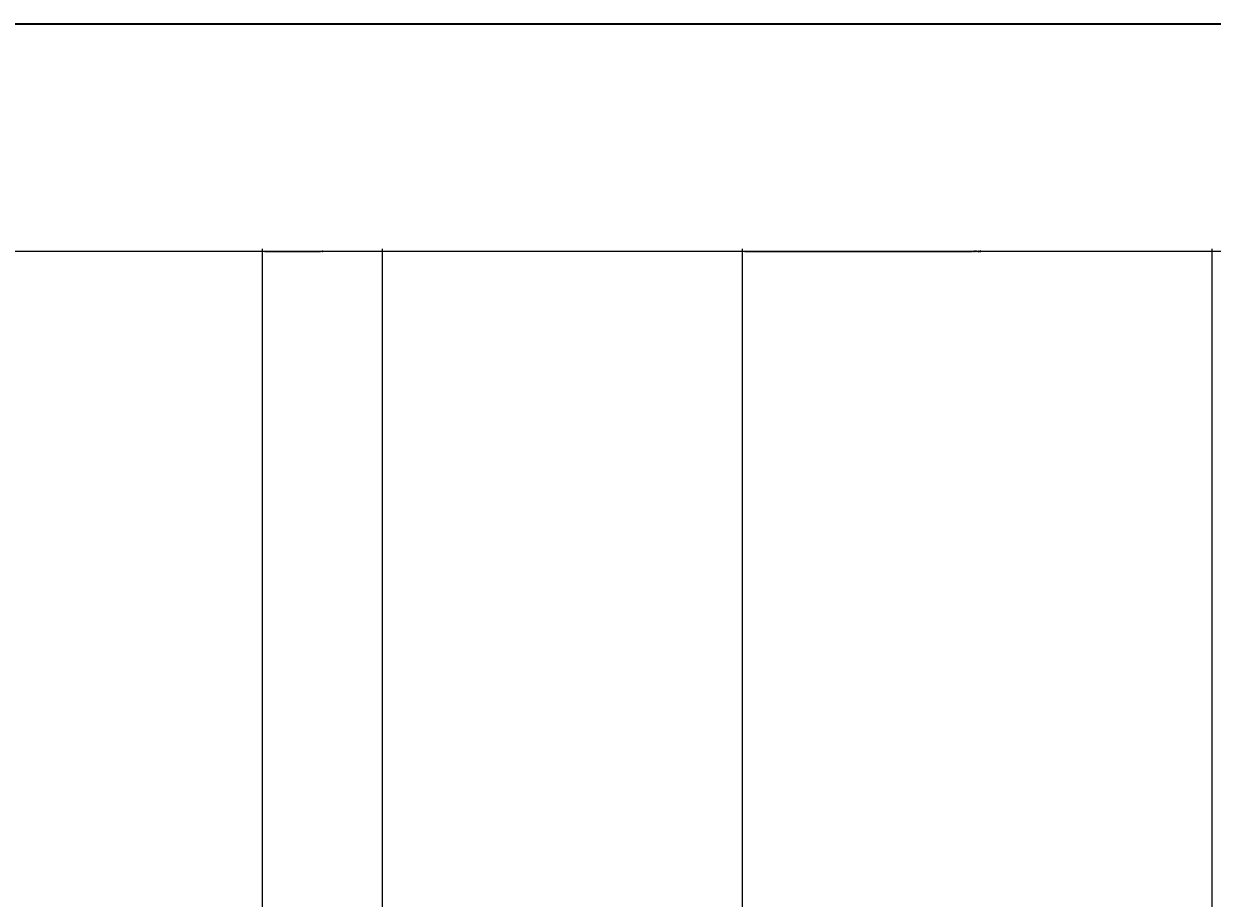
# Model space of a CAD drawing. Units: inches. Extents: x 1088 to 1703, y 668 to 1875.
# Tile 44 of 45: x 1497 to 1586, y 1809 to 1875. Entities that reach past the tile are written whole.
import ezdxf

# ---------------------------------------------------------------- set-up
doc = ezdxf.new("R2010")
doc.units = ezdxf.units.IN
doc.layers.add('A-ANNO-DIMS', color=2, linetype='Continuous', lineweight=18)
doc.layers.add('A-ANNO-TTLB', color=7, linetype='Continuous', lineweight=35)
doc.styles.get("Standard").update_dxf_attribs({"font": 'arial.ttf'})
doc.dimstyles.get("Standard").update_dxf_attribs({"dimtxt": 0.18, "dimasz": 0.18, "dimexe": 0.18, "dimexo": 0.0625, "dimgap": 0.09, "dimtad": 0, "dimtih": 1, "dimtoh": 1, "dimdec": 4, "dimzin": 0, "dimdsep": 46, "dimtxsty": 'Standard', "dimcen": 0.09, "dimadec": 0, "dimazin": 0, "dimtfac": 1, "dimtdec": 4, "dimtofl": 0, "dimtmove": 0, "dimatfit": 3, "dimfxl": 1, "dimtolj": 1, "dimtzin": 0, "dimarcsym": 0})

# ---------------------------------------------------------------- blocks, each defined once
blk = doc.blocks.new('*D28')
at = {"layer": 'A-ANNO-DIMS', "color": 0, "lineweight": -2, "transparency": 16777216}
for p, q in [((1170.345, 1803.621), (1170.345, 1857.788)), ((1170.525, 1857.608), (1408.147, 1857.608)), ((1646.563, 1857.608), (1408.941, 1857.608)), ((1646.743, 1745.552), (1646.743, 1857.788))]:
    blk.add_line(p, q, dxfattribs=at)
at = {"layer": 'A-ANNO-DIMS', "color": 0, "transparency": 16777216}
for points in [[(1170.525, 1857.638), (1170.525, 1857.578), (1170.345, 1857.608)], [(1646.563, 1857.638), (1646.563, 1857.578), (1646.743, 1857.608)]]:
    blk.add_solid(points, dxfattribs=at)
at = {"layer": 'Defpoints', "color": 0, "transparency": 16777216}
for p in [(1646.743, 1857.608), (1170.345, 1803.558), (1646.743, 1745.49)]:
    blk.add_point(p, dxfattribs=at)
at = {"layer": 'A-ANNO-DIMS', "color": 0, "transparency": 16777216, "insert": (1408.544, 1857.608), "char_height": 0.18, "attachment_point": 5}
blk.add_mtext('\\A1;476.4', dxfattribs=at)
blk = doc.blocks.new('*D32')
at = {"layer": 'A-ANNO-DIMS', "color": 0, "lineweight": -2, "transparency": 16777216}
for p, q in [((1550.595, 1373.121), (1550.595, 1857.788)), ((1550.775, 1857.608), (1567.825, 1857.608)), ((1585.665, 1857.608), (1568.614, 1857.608)), ((1585.845, 1360.983), (1585.845, 1857.788))]:
    blk.add_line(p, q, dxfattribs=at)
at = {"layer": 'A-ANNO-DIMS', "color": 0, "transparency": 16777216}
for points in [[(1550.775, 1857.638), (1550.775, 1857.578), (1550.595, 1857.608)], [(1585.665, 1857.638), (1585.665, 1857.578), (1585.845, 1857.608)]]:
    blk.add_solid(points, dxfattribs=at)
at = {"layer": 'Defpoints', "color": 0, "transparency": 16777216}
for p in [(1585.845, 1857.608), (1550.595, 1373.058), (1585.845, 1360.921)]:
    blk.add_point(p, dxfattribs=at)
at = {"layer": 'A-ANNO-DIMS', "color": 0, "transparency": 16777216, "insert": (1568.22, 1857.608), "char_height": 0.18, "attachment_point": 5}
blk.add_mtext('\\A1;35.25', dxfattribs=at)
blk = doc.blocks.new('*D33')
at = {"layer": 'A-ANNO-DIMS', "color": 0, "lineweight": -2, "transparency": 16777216}
for p, q in [((1514.595, 1355.648), (1514.595, 1857.788)), ((1514.775, 1857.608), (1518.946, 1857.608)), ((1523.415, 1857.608), (1519.244, 1857.608)), ((1523.595, 1331.121), (1523.595, 1857.788))]:
    blk.add_line(p, q, dxfattribs=at)
at = {"layer": 'A-ANNO-DIMS', "color": 0, "transparency": 16777216}
for points in [[(1514.775, 1857.638), (1514.775, 1857.578), (1514.595, 1857.608)], [(1523.415, 1857.638), (1523.415, 1857.578), (1523.595, 1857.608)]]:
    blk.add_solid(points, dxfattribs=at)
at = {"layer": 'Defpoints', "color": 0, "transparency": 16777216}
for p in [(1523.595, 1857.608), (1514.595, 1355.585), (1523.595, 1331.058)]:
    blk.add_point(p, dxfattribs=at)
at = {"layer": 'A-ANNO-DIMS', "color": 0, "transparency": 16777216, "insert": (1519.095, 1857.608), "char_height": 0.18, "attachment_point": 5}
blk.add_mtext('\\A1;9', dxfattribs=at)

msp = doc.modelspace()

# ---------------------------------------------------------------- linework, layer by layer
at = {"layer": 'A-ANNO-TTLB'}
msp.add_lwpolyline([(1088.369, 1874.677), (1703.181, 1874.677), (1703.181, 667.947), (1088.369, 667.947)], close=True, dxfattribs=at)

# ---------------------------------------------------------------- dimensions: what is measured, and where the dimension line sits
at = {"layer": 'A-ANNO-DIMS'}
for base, p1, p2, override, picture, middle in [((1646.743, 1857.608), (1170.345, 1803.558), (1646.743, 1745.49), {"dimdec": 1, "dimlfac": 1, "dimrnd": 0, "dimzin": 0, "dimdsep": 46, "dimlunit": 2}, '*D28', (1408.544, 1857.608)), ((1523.595, 1857.608), (1514.595, 1355.585), (1523.595, 1331.058), {"dimdec": 0, "dimlfac": 1, "dimrnd": 0, "dimzin": 0, "dimdsep": 46, "dimlunit": 2}, '*D33', (1519.095, 1857.608)), ((1585.845, 1857.608), (1550.595, 1373.058), (1585.845, 1360.921), {"dimdec": 2, "dimlfac": 1, "dimrnd": 0, "dimzin": 0, "dimdsep": 46, "dimlunit": 2}, '*D32', (1568.22, 1857.608))]:
    dim = msp.add_linear_dim(base=base, p1=p1, p2=p2, dimstyle='Standard', override=override, dxfattribs=at)
    dim.commit()
    dim.dimension.update_dxf_attribs({"geometry": picture, "text_midpoint": middle})

doc.saveas('drawing.dxf')
